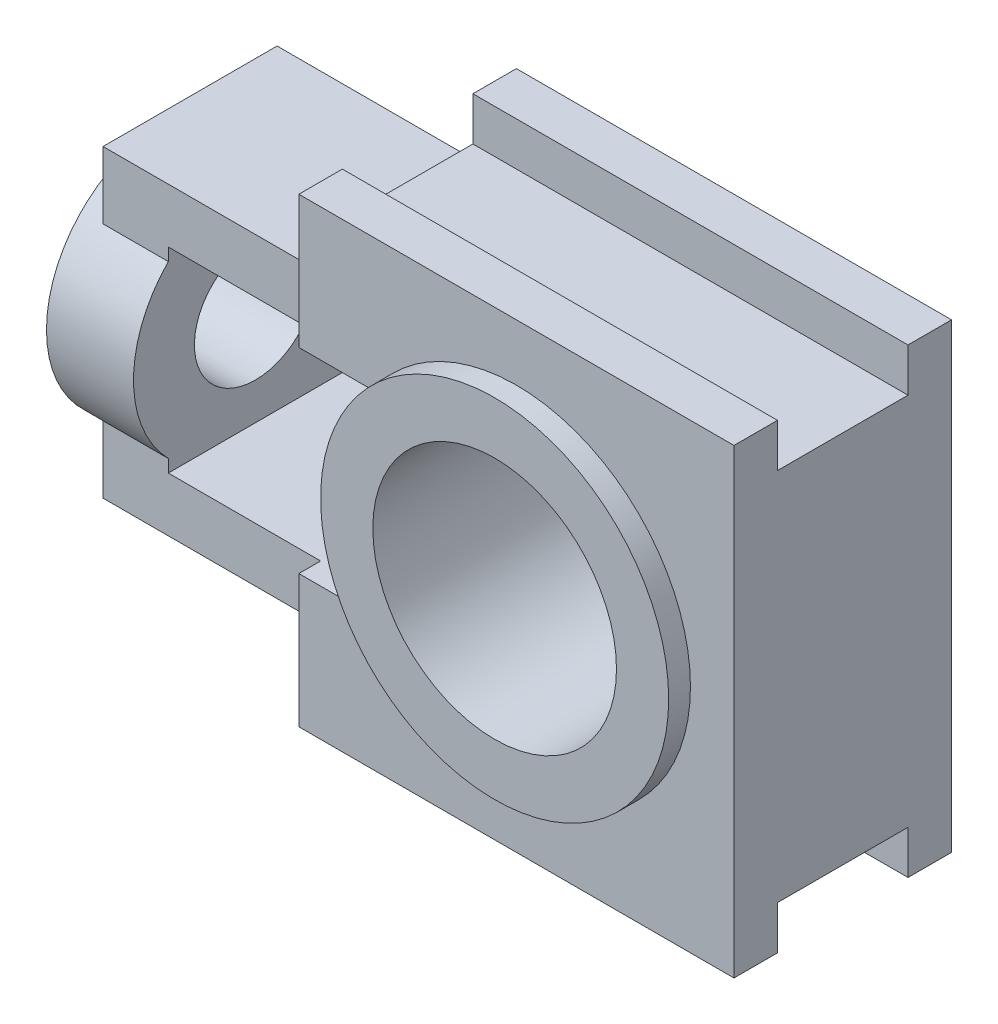
ISO-10303-21;
HEADER;
FILE_DESCRIPTION(('STEP AP214'),'2;1');
FILE_NAME('part.step','',(''),(''),'','','');
FILE_SCHEMA(('AUTOMOTIVE_DESIGN { 1 0 10303 214 1 1 1 1 }'));
ENDSEC;
DATA;
#1=APPLICATION_CONTEXT('core data for automotive mechanical design processes');
#2=APPLICATION_PROTOCOL_DEFINITION('international standard','automotive_design',2000,#1);
#3=PRODUCT_CONTEXT('',#1,'mechanical');
#4=PRODUCT('Part','Part','',(#3));
#5=PRODUCT_RELATED_PRODUCT_CATEGORY('part','',(#4));
#6=PRODUCT_DEFINITION_FORMATION('','',#4);
#7=PRODUCT_DEFINITION_CONTEXT('part definition',#1,'design');
#8=PRODUCT_DEFINITION('design','',#6,#7);
#9=PRODUCT_DEFINITION_SHAPE('','',#8);
#10=(LENGTH_UNIT() NAMED_UNIT(*) SI_UNIT(.MILLI.,.METRE.));
#11=(NAMED_UNIT(*) PLANE_ANGLE_UNIT() SI_UNIT($,.RADIAN.));
#12=(NAMED_UNIT(*) SI_UNIT($,.STERADIAN.) SOLID_ANGLE_UNIT());
#13=UNCERTAINTY_MEASURE_WITH_UNIT(LENGTH_MEASURE(1.E-05),#10,'distance_accuracy_value','');
#14=(GEOMETRIC_REPRESENTATION_CONTEXT(3) GLOBAL_UNCERTAINTY_ASSIGNED_CONTEXT((#13)) GLOBAL_UNIT_ASSIGNED_CONTEXT((#10,
#11,#12)) REPRESENTATION_CONTEXT('',''));
#15=CARTESIAN_POINT('',(0.,0.,0.));
#16=DIRECTION('',(0.,0.,1.));
#17=DIRECTION('',(1.,0.,0.));
#18=AXIS2_PLACEMENT_3D('',#15,#16,#17);
#19=CARTESIAN_POINT('',(0.,0.,20.));
#20=DIRECTION('',(0.,0.,-1.));
#21=DIRECTION('',(-1.,0.,0.));
#22=AXIS2_PLACEMENT_3D('',#19,#20,#21);
#23=PLANE('',#22);
#24=DIRECTION('',(1.,0.,0.));
#25=VECTOR('',#24,1.);
#26=CARTESIAN_POINT('',(-105.,19.5959179422654,20.));
#27=LINE('',#26,#25);
#28=CARTESIAN_POINT('',(-85.,19.5959179422654,20.));
#29=VERTEX_POINT('',#28);
#30=CARTESIAN_POINT('',(-100.,19.5959179422654,20.));
#31=VERTEX_POINT('',#30);
#32=EDGE_CURVE('E348',#29,#31,#27,.F.);
#33=ORIENTED_EDGE('',*,*,#32,.F.);
#34=DIRECTION('',(0.,1.,0.));
#35=VECTOR('',#34,1.);
#36=CARTESIAN_POINT('',(-85.,0.,20.));
#37=LINE('',#36,#35);
#38=CARTESIAN_POINT('',(-85.,22.5,20.));
#39=VERTEX_POINT('',#38);
#40=EDGE_CURVE('E291',#29,#39,#37,.T.);
#41=ORIENTED_EDGE('',*,*,#40,.T.);
#42=DIRECTION('',(1.,0.,0.));
#43=VECTOR('',#42,1.);
#44=CARTESIAN_POINT('',(0.,22.5,20.));
#45=LINE('',#44,#43);
#46=CARTESIAN_POINT('',(-50.,22.5,20.));
#47=VERTEX_POINT('',#46);
#48=EDGE_CURVE('E331',#39,#47,#45,.T.);
#49=ORIENTED_EDGE('',*,*,#48,.T.);
#50=DIRECTION('',(0.,1.,0.));
#51=VECTOR('',#50,1.);
#52=CARTESIAN_POINT('',(-50.,35.,20.));
#53=LINE('',#52,#51);
#54=CARTESIAN_POINT('',(-50.,35.,20.));
#55=VERTEX_POINT('',#54);
#56=EDGE_CURVE('E414',#47,#55,#53,.T.);
#57=ORIENTED_EDGE('',*,*,#56,.T.);
#58=DIRECTION('',(-1.,0.,0.));
#59=VECTOR('',#58,1.);
#60=CARTESIAN_POINT('',(-50.,35.,20.));
#61=LINE('',#60,#59);
#62=CARTESIAN_POINT('',(-100.,35.,20.));
#63=VERTEX_POINT('',#62);
#64=EDGE_CURVE('E413',#55,#63,#61,.T.);
#65=ORIENTED_EDGE('',*,*,#64,.T.);
#66=DIRECTION('',(0.,-1.,0.));
#67=VECTOR('',#66,1.);
#68=CARTESIAN_POINT('',(-100.,35.,20.));
#69=LINE('',#68,#67);
#70=EDGE_CURVE('E417',#63,#31,#69,.T.);
#71=ORIENTED_EDGE('',*,*,#70,.T.);
#72=EDGE_LOOP('',(#33,#41,#49,#57,#65,#71));
#73=FACE_BOUND('',#72,.T.);
#74=ADVANCED_FACE('F44',(#73),#23,.F.);
#75=CARTESIAN_POINT('',(0.,0.,-20.));
#76=DIRECTION('',(0.,0.,-1.));
#77=DIRECTION('',(-1.,0.,0.));
#78=AXIS2_PLACEMENT_3D('',#75,#76,#77);
#79=PLANE('',#78);
#80=DIRECTION('',(0.,1.,0.));
#81=VECTOR('',#80,1.);
#82=CARTESIAN_POINT('',(-85.,0.,-20.));
#83=LINE('',#82,#81);
#84=CARTESIAN_POINT('',(-85.,19.5959179422654,-20.));
#85=VERTEX_POINT('',#84);
#86=CARTESIAN_POINT('',(-85.,22.5,-20.));
#87=VERTEX_POINT('',#86);
#88=EDGE_CURVE('E301',#85,#87,#83,.T.);
#89=ORIENTED_EDGE('',*,*,#88,.F.);
#90=DIRECTION('',(1.,0.,0.));
#91=VECTOR('',#90,1.);
#92=CARTESIAN_POINT('',(-105.,19.5959179422654,-20.));
#93=LINE('',#92,#91);
#94=CARTESIAN_POINT('',(-100.,19.5959179422654,-20.));
#95=VERTEX_POINT('',#94);
#96=EDGE_CURVE('E11',#85,#95,#93,.F.);
#97=ORIENTED_EDGE('',*,*,#96,.T.);
#98=DIRECTION('',(0.,-1.,0.));
#99=VECTOR('',#98,1.);
#100=CARTESIAN_POINT('',(-100.,35.,-20.));
#101=LINE('',#100,#99);
#102=CARTESIAN_POINT('',(-100.,35.,-20.));
#103=VERTEX_POINT('',#102);
#104=EDGE_CURVE('E427',#103,#95,#101,.T.);
#105=ORIENTED_EDGE('',*,*,#104,.F.);
#106=DIRECTION('',(-1.,0.,0.));
#107=VECTOR('',#106,1.);
#108=CARTESIAN_POINT('',(-50.,35.,-20.));
#109=LINE('',#108,#107);
#110=CARTESIAN_POINT('',(-50.,35.,-20.));
#111=VERTEX_POINT('',#110);
#112=EDGE_CURVE('E426',#111,#103,#109,.T.);
#113=ORIENTED_EDGE('',*,*,#112,.F.);
#114=DIRECTION('',(0.,1.,0.));
#115=VECTOR('',#114,1.);
#116=CARTESIAN_POINT('',(-50.,35.,-20.));
#117=LINE('',#116,#115);
#118=CARTESIAN_POINT('',(-50.,22.5,-20.));
#119=VERTEX_POINT('',#118);
#120=EDGE_CURVE('E390',#119,#111,#117,.T.);
#121=ORIENTED_EDGE('',*,*,#120,.F.);
#122=DIRECTION('',(1.,0.,0.));
#123=VECTOR('',#122,1.);
#124=CARTESIAN_POINT('',(0.,22.5,-20.));
#125=LINE('',#124,#123);
#126=EDGE_CURVE('E327',#87,#119,#125,.T.);
#127=ORIENTED_EDGE('',*,*,#126,.F.);
#128=EDGE_LOOP('',(#89,#97,#105,#113,#121,#127));
#129=FACE_BOUND('',#128,.T.);
#130=ADVANCED_FACE('F524',(#129),#79,.T.);
#131=CARTESIAN_POINT('',(-50.,-53.,25.));
#132=DIRECTION('',(1.,0.,0.));
#133=DIRECTION('',(0.,0.,-1.));
#134=AXIS2_PLACEMENT_3D('',#131,#132,#133);
#135=PLANE('',#134);
#136=DIRECTION('',(0.,-1.,0.));
#137=VECTOR('',#136,1.);
#138=CARTESIAN_POINT('',(-50.,-53.,-25.));
#139=LINE('',#138,#137);
#140=CARTESIAN_POINT('',(-50.,53.,-25.));
#141=VERTEX_POINT('',#140);
#142=CARTESIAN_POINT('',(-50.,22.5,-25.));
#143=VERTEX_POINT('',#142);
#144=EDGE_CURVE('E467',#141,#143,#139,.T.);
#145=ORIENTED_EDGE('',*,*,#144,.T.);
#146=DIRECTION('',(0.,0.,1.));
#147=VECTOR('',#146,1.);
#148=CARTESIAN_POINT('',(-50.,22.5,25.));
#149=LINE('',#148,#147);
#150=EDGE_CURVE('E324',#143,#119,#149,.T.);
#151=ORIENTED_EDGE('',*,*,#150,.T.);
#152=ORIENTED_EDGE('',*,*,#120,.T.);
#153=DIRECTION('',(0.,0.,-1.));
#154=VECTOR('',#153,1.);
#155=CARTESIAN_POINT('',(-50.,35.,20.));
#156=LINE('',#155,#154);
#157=EDGE_CURVE('E444',#55,#111,#156,.T.);
#158=ORIENTED_EDGE('',*,*,#157,.F.);
#159=ORIENTED_EDGE('',*,*,#56,.F.);
#160=CARTESIAN_POINT('',(-50.,22.5,25.));
#161=VERTEX_POINT('',#160);
#162=EDGE_CURVE('E328',#47,#161,#149,.T.);
#163=ORIENTED_EDGE('',*,*,#162,.T.);
#164=DIRECTION('',(0.,-1.,0.));
#165=VECTOR('',#164,1.);
#166=CARTESIAN_POINT('',(-50.,-53.,25.));
#167=LINE('',#166,#165);
#168=CARTESIAN_POINT('',(-50.,53.,25.));
#169=VERTEX_POINT('',#168);
#170=EDGE_CURVE('E454',#169,#161,#167,.T.);
#171=ORIENTED_EDGE('',*,*,#170,.F.);
#172=DIRECTION('',(0.,0.,-1.));
#173=VECTOR('',#172,1.);
#174=CARTESIAN_POINT('',(-50.,53.,25.));
#175=LINE('',#174,#173);
#176=CARTESIAN_POINT('',(-50.,53.,15.));
#177=VERTEX_POINT('',#176);
#178=EDGE_CURVE('E479',#169,#177,#175,.T.);
#179=ORIENTED_EDGE('',*,*,#178,.T.);
#180=DIRECTION('',(0.,1.,0.));
#181=VECTOR('',#180,1.);
#182=CARTESIAN_POINT('',(-50.,53.,15.));
#183=LINE('',#182,#181);
#184=CARTESIAN_POINT('',(-50.,43.,15.));
#185=VERTEX_POINT('',#184);
#186=EDGE_CURVE('E374',#185,#177,#183,.T.);
#187=ORIENTED_EDGE('',*,*,#186,.F.);
#188=DIRECTION('',(0.,0.,1.));
#189=VECTOR('',#188,1.);
#190=CARTESIAN_POINT('',(-50.,43.,-15.));
#191=LINE('',#190,#189);
#192=CARTESIAN_POINT('',(-50.,43.,-15.));
#193=VERTEX_POINT('',#192);
#194=EDGE_CURVE('E371',#193,#185,#191,.T.);
#195=ORIENTED_EDGE('',*,*,#194,.F.);
#196=DIRECTION('',(0.,-1.,0.));
#197=VECTOR('',#196,1.);
#198=CARTESIAN_POINT('',(-50.,53.,-15.));
#199=LINE('',#198,#197);
#200=CARTESIAN_POINT('',(-50.,53.,-15.));
#201=VERTEX_POINT('',#200);
#202=EDGE_CURVE('E369',#201,#193,#199,.T.);
#203=ORIENTED_EDGE('',*,*,#202,.F.);
#204=EDGE_CURVE('E476',#201,#141,#175,.T.);
#205=ORIENTED_EDGE('',*,*,#204,.T.);
#206=EDGE_LOOP('',(#145,#151,#152,#158,#159,#163,#171,#179,#187,#195,#203,#205));
#207=FACE_BOUND('',#206,.T.);
#208=ADVANCED_FACE('F590',(#207),#135,.F.);
#209=CARTESIAN_POINT('',(-100.,35.,20.));
#210=DIRECTION('',(1.,0.,0.));
#211=DIRECTION('',(0.,0.,-1.));
#212=AXIS2_PLACEMENT_3D('',#209,#210,#211);
#213=PLANE('',#212);
#214=CARTESIAN_POINT('',(-100.,0.,0.));
#215=DIRECTION('',(1.,0.,0.));
#216=DIRECTION('',(0.,0.,-1.));
#217=AXIS2_PLACEMENT_3D('',#214,#215,#216);
#218=CIRCLE('',#217,28.);
#219=CARTESIAN_POINT('',(-100.,-19.5959179422654,-20.));
#220=VERTEX_POINT('',#219);
#221=CARTESIAN_POINT('',(-100.,-19.5959179422654,20.));
#222=VERTEX_POINT('',#221);
#223=EDGE_CURVE('E344',#220,#222,#218,.F.);
#224=ORIENTED_EDGE('',*,*,#223,.F.);
#225=CARTESIAN_POINT('',(-100.,-35.,-20.));
#226=VERTEX_POINT('',#225);
#227=EDGE_CURVE('E428',#220,#226,#101,.T.);
#228=ORIENTED_EDGE('',*,*,#227,.T.);
#229=DIRECTION('',(0.,0.,-1.));
#230=VECTOR('',#229,1.);
#231=CARTESIAN_POINT('',(-100.,-35.,20.));
#232=LINE('',#231,#230);
#233=CARTESIAN_POINT('',(-100.,-35.,20.));
#234=VERTEX_POINT('',#233);
#235=EDGE_CURVE('E440',#234,#226,#232,.T.);
#236=ORIENTED_EDGE('',*,*,#235,.F.);
#237=EDGE_CURVE('E418',#222,#234,#69,.T.);
#238=ORIENTED_EDGE('',*,*,#237,.F.);
#239=EDGE_LOOP('',(#224,#228,#236,#238));
#240=FACE_BOUND('',#239,.T.);
#241=ADVANCED_FACE('F505',(#240),#213,.F.);
#242=DIRECTION('',(-1.,0.,0.));
#243=VECTOR('',#242,1.);
#244=CARTESIAN_POINT('',(0.,-22.5,20.));
#245=LINE('',#244,#243);
#246=CARTESIAN_POINT('',(-50.,-22.5,20.));
#247=VERTEX_POINT('',#246);
#248=CARTESIAN_POINT('',(-85.,-22.5,20.));
#249=VERTEX_POINT('',#248);
#250=EDGE_CURVE('E319',#247,#249,#245,.T.);
#251=ORIENTED_EDGE('',*,*,#250,.T.);
#252=CARTESIAN_POINT('',(-85.,-19.5959179422654,20.));
#253=VERTEX_POINT('',#252);
#254=EDGE_CURVE('E308',#249,#253,#37,.T.);
#255=ORIENTED_EDGE('',*,*,#254,.T.);
#256=DIRECTION('',(1.,0.,0.));
#257=VECTOR('',#256,1.);
#258=CARTESIAN_POINT('',(-105.,-19.5959179422654,20.));
#259=LINE('',#258,#257);
#260=EDGE_CURVE('E347',#222,#253,#259,.T.);
#261=ORIENTED_EDGE('',*,*,#260,.F.);
#262=ORIENTED_EDGE('',*,*,#237,.T.);
#263=DIRECTION('',(1.,0.,0.));
#264=VECTOR('',#263,1.);
#265=CARTESIAN_POINT('',(-50.,-35.,20.));
#266=LINE('',#265,#264);
#267=CARTESIAN_POINT('',(-50.,-35.,20.));
#268=VERTEX_POINT('',#267);
#269=EDGE_CURVE('E419',#234,#268,#266,.T.);
#270=ORIENTED_EDGE('',*,*,#269,.T.);
#271=EDGE_CURVE('E407',#268,#247,#53,.T.);
#272=ORIENTED_EDGE('',*,*,#271,.T.);
#273=EDGE_LOOP('',(#251,#255,#261,#262,#270,#272));
#274=FACE_BOUND('',#273,.T.);
#275=ADVANCED_FACE('F507',(#274),#23,.F.);
#276=CARTESIAN_POINT('',(-85.,-22.5,-20.));
#277=VERTEX_POINT('',#276);
#278=CARTESIAN_POINT('',(-85.,-19.5959179422654,-20.));
#279=VERTEX_POINT('',#278);
#280=EDGE_CURVE('E306',#277,#279,#83,.T.);
#281=ORIENTED_EDGE('',*,*,#280,.F.);
#282=DIRECTION('',(-1.,0.,0.));
#283=VECTOR('',#282,1.);
#284=CARTESIAN_POINT('',(0.,-22.5,-20.));
#285=LINE('',#284,#283);
#286=CARTESIAN_POINT('',(-50.,-22.5,-20.));
#287=VERTEX_POINT('',#286);
#288=EDGE_CURVE('E314',#287,#277,#285,.T.);
#289=ORIENTED_EDGE('',*,*,#288,.F.);
#290=CARTESIAN_POINT('',(-50.,-35.,-20.));
#291=VERTEX_POINT('',#290);
#292=EDGE_CURVE('E421',#291,#287,#117,.T.);
#293=ORIENTED_EDGE('',*,*,#292,.F.);
#294=DIRECTION('',(1.,0.,0.));
#295=VECTOR('',#294,1.);
#296=CARTESIAN_POINT('',(-50.,-35.,-20.));
#297=LINE('',#296,#295);
#298=EDGE_CURVE('E435',#226,#291,#297,.T.);
#299=ORIENTED_EDGE('',*,*,#298,.F.);
#300=ORIENTED_EDGE('',*,*,#227,.F.);
#301=DIRECTION('',(1.,0.,0.));
#302=VECTOR('',#301,1.);
#303=CARTESIAN_POINT('',(-105.,-19.5959179422654,-20.));
#304=LINE('',#303,#302);
#305=EDGE_CURVE('E52',#220,#279,#304,.T.);
#306=ORIENTED_EDGE('',*,*,#305,.T.);
#307=EDGE_LOOP('',(#281,#289,#293,#299,#300,#306));
#308=FACE_BOUND('',#307,.T.);
#309=ADVANCED_FACE('F489',(#308),#79,.T.);
#310=CARTESIAN_POINT('',(-50.,53.,25.));
#311=DIRECTION('',(0.,-1.,0.));
#312=DIRECTION('',(0.,0.,-1.));
#313=AXIS2_PLACEMENT_3D('',#310,#311,#312);
#314=PLANE('',#313);
#315=ORIENTED_EDGE('',*,*,#204,.F.);
#316=DIRECTION('',(-1.,0.,0.));
#317=VECTOR('',#316,1.);
#318=CARTESIAN_POINT('',(81.6227766016838,53.,-15.));
#319=LINE('',#318,#317);
#320=CARTESIAN_POINT('',(50.,53.,-15.));
#321=VERTEX_POINT('',#320);
#322=EDGE_CURVE('E368',#321,#201,#319,.T.);
#323=ORIENTED_EDGE('',*,*,#322,.F.);
#324=DIRECTION('',(0.,0.,-1.));
#325=VECTOR('',#324,1.);
#326=CARTESIAN_POINT('',(50.,53.,25.));
#327=LINE('',#326,#325);
#328=CARTESIAN_POINT('',(50.,53.,-25.));
#329=VERTEX_POINT('',#328);
#330=EDGE_CURVE('E485',#321,#329,#327,.T.);
#331=ORIENTED_EDGE('',*,*,#330,.T.);
#332=DIRECTION('',(-1.,0.,0.));
#333=VECTOR('',#332,1.);
#334=CARTESIAN_POINT('',(-50.,53.,-25.));
#335=LINE('',#334,#333);
#336=EDGE_CURVE('E465',#329,#141,#335,.T.);
#337=ORIENTED_EDGE('',*,*,#336,.T.);
#338=EDGE_LOOP('',(#315,#323,#331,#337));
#339=FACE_BOUND('',#338,.T.);
#340=ADVANCED_FACE('F598',(#339),#314,.F.);
#341=CARTESIAN_POINT('',(-50.,-53.,25.));
#342=DIRECTION('',(0.,1.,0.));
#343=DIRECTION('',(0.,0.,1.));
#344=AXIS2_PLACEMENT_3D('',#341,#342,#343);
#345=PLANE('',#344);
#346=DIRECTION('',(0.,0.,-1.));
#347=VECTOR('',#346,1.);
#348=CARTESIAN_POINT('',(50.,-53.,25.));
#349=LINE('',#348,#347);
#350=CARTESIAN_POINT('',(50.,-53.,-15.));
#351=VERTEX_POINT('',#350);
#352=CARTESIAN_POINT('',(50.,-53.,-25.));
#353=VERTEX_POINT('',#352);
#354=EDGE_CURVE('E459',#351,#353,#349,.T.);
#355=ORIENTED_EDGE('',*,*,#354,.F.);
#356=DIRECTION('',(-1.,0.,0.));
#357=VECTOR('',#356,1.);
#358=CARTESIAN_POINT('',(81.6227766016838,-53.,-15.));
#359=LINE('',#358,#357);
#360=CARTESIAN_POINT('',(-50.,-53.,-15.));
#361=VERTEX_POINT('',#360);
#362=EDGE_CURVE('E393',#351,#361,#359,.T.);
#363=ORIENTED_EDGE('',*,*,#362,.T.);
#364=DIRECTION('',(0.,0.,-1.));
#365=VECTOR('',#364,1.);
#366=CARTESIAN_POINT('',(-50.,-53.,25.));
#367=LINE('',#366,#365);
#368=CARTESIAN_POINT('',(-50.,-53.,-25.));
#369=VERTEX_POINT('',#368);
#370=EDGE_CURVE('E475',#361,#369,#367,.T.);
#371=ORIENTED_EDGE('',*,*,#370,.T.);
#372=DIRECTION('',(1.,0.,0.));
#373=VECTOR('',#372,1.);
#374=CARTESIAN_POINT('',(-50.,-53.,-25.));
#375=LINE('',#374,#373);
#376=EDGE_CURVE('E452',#369,#353,#375,.T.);
#377=ORIENTED_EDGE('',*,*,#376,.T.);
#378=EDGE_LOOP('',(#355,#363,#371,#377));
#379=FACE_BOUND('',#378,.T.);
#380=ADVANCED_FACE('F553',(#379),#345,.F.);
#381=CARTESIAN_POINT('',(50.,-53.,25.));
#382=DIRECTION('',(-1.,0.,0.));
#383=DIRECTION('',(0.,0.,1.));
#384=AXIS2_PLACEMENT_3D('',#381,#382,#383);
#385=PLANE('',#384);
#386=ORIENTED_EDGE('',*,*,#330,.F.);
#387=DIRECTION('',(0.,1.,0.));
#388=VECTOR('',#387,1.);
#389=CARTESIAN_POINT('',(50.,53.,-15.));
#390=LINE('',#389,#388);
#391=CARTESIAN_POINT('',(50.,43.,-15.));
#392=VERTEX_POINT('',#391);
#393=EDGE_CURVE('E364',#392,#321,#390,.T.);
#394=ORIENTED_EDGE('',*,*,#393,.F.);
#395=DIRECTION('',(0.,0.,-1.));
#396=VECTOR('',#395,1.);
#397=CARTESIAN_POINT('',(50.,43.,-15.));
#398=LINE('',#397,#396);
#399=CARTESIAN_POINT('',(50.,43.,15.));
#400=VERTEX_POINT('',#399);
#401=EDGE_CURVE('E366',#400,#392,#398,.T.);
#402=ORIENTED_EDGE('',*,*,#401,.F.);
#403=DIRECTION('',(0.,-1.,0.));
#404=VECTOR('',#403,1.);
#405=CARTESIAN_POINT('',(50.,53.,15.));
#406=LINE('',#405,#404);
#407=CARTESIAN_POINT('',(50.,53.,15.));
#408=VERTEX_POINT('',#407);
#409=EDGE_CURVE('E361',#408,#400,#406,.T.);
#410=ORIENTED_EDGE('',*,*,#409,.F.);
#411=CARTESIAN_POINT('',(50.,53.,25.));
#412=VERTEX_POINT('',#411);
#413=EDGE_CURVE('E362',#412,#408,#327,.T.);
#414=ORIENTED_EDGE('',*,*,#413,.F.);
#415=DIRECTION('',(0.,1.,0.));
#416=VECTOR('',#415,1.);
#417=CARTESIAN_POINT('',(50.,-53.,25.));
#418=LINE('',#417,#416);
#419=CARTESIAN_POINT('',(50.,-53.,25.));
#420=VERTEX_POINT('',#419);
#421=EDGE_CURVE('E450',#420,#412,#418,.T.);
#422=ORIENTED_EDGE('',*,*,#421,.F.);
#423=CARTESIAN_POINT('',(50.,-53.,15.));
#424=VERTEX_POINT('',#423);
#425=EDGE_CURVE('E473',#420,#424,#349,.T.);
#426=ORIENTED_EDGE('',*,*,#425,.T.);
#427=DIRECTION('',(0.,-1.,0.));
#428=VECTOR('',#427,1.);
#429=CARTESIAN_POINT('',(50.,-53.,15.));
#430=LINE('',#429,#428);
#431=CARTESIAN_POINT('',(50.,-43.,15.));
#432=VERTEX_POINT('',#431);
#433=EDGE_CURVE('E375',#432,#424,#430,.T.);
#434=ORIENTED_EDGE('',*,*,#433,.F.);
#435=DIRECTION('',(0.,0.,1.));
#436=VECTOR('',#435,1.);
#437=CARTESIAN_POINT('',(50.,-43.,-15.));
#438=LINE('',#437,#436);
#439=CARTESIAN_POINT('',(50.,-43.,-15.));
#440=VERTEX_POINT('',#439);
#441=EDGE_CURVE('E389',#440,#432,#438,.T.);
#442=ORIENTED_EDGE('',*,*,#441,.F.);
#443=DIRECTION('',(0.,1.,0.));
#444=VECTOR('',#443,1.);
#445=CARTESIAN_POINT('',(50.,-53.,-15.));
#446=LINE('',#445,#444);
#447=EDGE_CURVE('E388',#351,#440,#446,.T.);
#448=ORIENTED_EDGE('',*,*,#447,.F.);
#449=ORIENTED_EDGE('',*,*,#354,.T.);
#450=DIRECTION('',(0.,1.,0.));
#451=VECTOR('',#450,1.);
#452=CARTESIAN_POINT('',(50.,-53.,-25.));
#453=LINE('',#452,#451);
#454=EDGE_CURVE('E448',#353,#329,#453,.T.);
#455=ORIENTED_EDGE('',*,*,#454,.T.);
#456=EDGE_LOOP('',(#386,#394,#402,#410,#414,#422,#426,#434,#442,#448,#449,#455));
#457=FACE_BOUND('',#456,.T.);
#458=ADVANCED_FACE('F50',(#457),#385,.F.);
#459=ORIENTED_EDGE('',*,*,#413,.T.);
#460=DIRECTION('',(-1.,0.,0.));
#461=VECTOR('',#460,1.);
#462=CARTESIAN_POINT('',(81.6227766016838,53.,15.));
#463=LINE('',#462,#461);
#464=EDGE_CURVE('E377',#408,#177,#463,.T.);
#465=ORIENTED_EDGE('',*,*,#464,.T.);
#466=ORIENTED_EDGE('',*,*,#178,.F.);
#467=DIRECTION('',(-1.,0.,0.));
#468=VECTOR('',#467,1.);
#469=CARTESIAN_POINT('',(-50.,53.,25.));
#470=LINE('',#469,#468);
#471=EDGE_CURVE('E447',#412,#169,#470,.T.);
#472=ORIENTED_EDGE('',*,*,#471,.F.);
#473=EDGE_LOOP('',(#459,#465,#466,#472));
#474=FACE_BOUND('',#473,.T.);
#475=ADVANCED_FACE('F582',(#474),#314,.F.);
#476=CARTESIAN_POINT('',(-50.,-22.5,25.));
#477=VERTEX_POINT('',#476);
#478=CARTESIAN_POINT('',(-50.,-53.,25.));
#479=VERTEX_POINT('',#478);
#480=EDGE_CURVE('E453',#477,#479,#167,.T.);
#481=ORIENTED_EDGE('',*,*,#480,.F.);
#482=DIRECTION('',(0.,0.,-1.));
#483=VECTOR('',#482,1.);
#484=CARTESIAN_POINT('',(-50.,-22.5,25.));
#485=LINE('',#484,#483);
#486=EDGE_CURVE('E312',#477,#247,#485,.T.);
#487=ORIENTED_EDGE('',*,*,#486,.T.);
#488=ORIENTED_EDGE('',*,*,#271,.F.);
#489=DIRECTION('',(0.,0.,-1.));
#490=VECTOR('',#489,1.);
#491=CARTESIAN_POINT('',(-50.,-35.,20.));
#492=LINE('',#491,#490);
#493=EDGE_CURVE('E425',#268,#291,#492,.T.);
#494=ORIENTED_EDGE('',*,*,#493,.T.);
#495=ORIENTED_EDGE('',*,*,#292,.T.);
#496=CARTESIAN_POINT('',(-50.,-22.5,-25.));
#497=VERTEX_POINT('',#496);
#498=EDGE_CURVE('E313',#287,#497,#485,.T.);
#499=ORIENTED_EDGE('',*,*,#498,.T.);
#500=EDGE_CURVE('E462',#497,#369,#139,.T.);
#501=ORIENTED_EDGE('',*,*,#500,.T.);
#502=ORIENTED_EDGE('',*,*,#370,.F.);
#503=DIRECTION('',(0.,-1.,0.));
#504=VECTOR('',#503,1.);
#505=CARTESIAN_POINT('',(-50.,-53.,-15.));
#506=LINE('',#505,#504);
#507=CARTESIAN_POINT('',(-50.,-43.,-15.));
#508=VERTEX_POINT('',#507);
#509=EDGE_CURVE('E399',#508,#361,#506,.T.);
#510=ORIENTED_EDGE('',*,*,#509,.F.);
#511=DIRECTION('',(0.,0.,-1.));
#512=VECTOR('',#511,1.);
#513=CARTESIAN_POINT('',(-50.,-43.,-15.));
#514=LINE('',#513,#512);
#515=CARTESIAN_POINT('',(-50.,-43.,15.));
#516=VERTEX_POINT('',#515);
#517=EDGE_CURVE('E397',#516,#508,#514,.T.);
#518=ORIENTED_EDGE('',*,*,#517,.F.);
#519=DIRECTION('',(0.,1.,0.));
#520=VECTOR('',#519,1.);
#521=CARTESIAN_POINT('',(-50.,-53.,15.));
#522=LINE('',#521,#520);
#523=CARTESIAN_POINT('',(-50.,-53.,15.));
#524=VERTEX_POINT('',#523);
#525=EDGE_CURVE('E391',#524,#516,#522,.T.);
#526=ORIENTED_EDGE('',*,*,#525,.F.);
#527=EDGE_CURVE('E474',#479,#524,#367,.T.);
#528=ORIENTED_EDGE('',*,*,#527,.F.);
#529=EDGE_LOOP('',(#481,#487,#488,#494,#495,#499,#501,#502,#510,#518,#526,#528));
#530=FACE_BOUND('',#529,.T.);
#531=ADVANCED_FACE('F531',(#530),#135,.F.);
#532=ORIENTED_EDGE('',*,*,#527,.T.);
#533=DIRECTION('',(-1.,0.,0.));
#534=VECTOR('',#533,1.);
#535=CARTESIAN_POINT('',(81.6227766016838,-53.,15.));
#536=LINE('',#535,#534);
#537=EDGE_CURVE('E402',#424,#524,#536,.T.);
#538=ORIENTED_EDGE('',*,*,#537,.F.);
#539=ORIENTED_EDGE('',*,*,#425,.F.);
#540=DIRECTION('',(1.,0.,0.));
#541=VECTOR('',#540,1.);
#542=CARTESIAN_POINT('',(-50.,-53.,25.));
#543=LINE('',#542,#541);
#544=EDGE_CURVE('E460',#479,#420,#543,.T.);
#545=ORIENTED_EDGE('',*,*,#544,.F.);
#546=EDGE_LOOP('',(#532,#538,#539,#545));
#547=FACE_BOUND('',#546,.T.);
#548=ADVANCED_FACE('F574',(#547),#345,.F.);
#549=CARTESIAN_POINT('',(0.,0.,25.));
#550=DIRECTION('',(0.,0.,-1.));
#551=DIRECTION('',(-1.,0.,0.));
#552=AXIS2_PLACEMENT_3D('',#549,#550,#551);
#553=PLANE('',#552);
#554=ORIENTED_EDGE('',*,*,#170,.T.);
#555=DIRECTION('',(1.,0.,0.));
#556=VECTOR('',#555,1.);
#557=CARTESIAN_POINT('',(0.,22.5,25.));
#558=LINE('',#557,#556);
#559=CARTESIAN_POINT('',(-33.0718913883074,22.5,25.));
#560=VERTEX_POINT('',#559);
#561=EDGE_CURVE('E332',#161,#560,#558,.T.);
#562=ORIENTED_EDGE('',*,*,#561,.T.);
#563=CARTESIAN_POINT('',(0.,0.,25.));
#564=DIRECTION('',(0.,0.,-1.));
#565=DIRECTION('',(-1.,0.,0.));
#566=AXIS2_PLACEMENT_3D('',#563,#564,#565);
#567=CIRCLE('',#566,40.);
#568=CARTESIAN_POINT('',(-33.0718913883074,-22.5,25.));
#569=VERTEX_POINT('',#568);
#570=EDGE_CURVE('E359',#569,#560,#567,.F.);
#571=ORIENTED_EDGE('',*,*,#570,.F.);
#572=DIRECTION('',(-1.,0.,0.));
#573=VECTOR('',#572,1.);
#574=CARTESIAN_POINT('',(0.,-22.5,25.));
#575=LINE('',#574,#573);
#576=EDGE_CURVE('E320',#569,#477,#575,.T.);
#577=ORIENTED_EDGE('',*,*,#576,.T.);
#578=ORIENTED_EDGE('',*,*,#480,.T.);
#579=ORIENTED_EDGE('',*,*,#544,.T.);
#580=ORIENTED_EDGE('',*,*,#421,.T.);
#581=ORIENTED_EDGE('',*,*,#471,.T.);
#582=EDGE_LOOP('',(#554,#562,#571,#577,#578,#579,#580,#581));
#583=FACE_BOUND('',#582,.T.);
#584=ADVANCED_FACE('F540',(#583),#553,.F.);
#585=CARTESIAN_POINT('',(0.,0.,-25.));
#586=DIRECTION('',(0.,0.,-1.));
#587=DIRECTION('',(-1.,0.,0.));
#588=AXIS2_PLACEMENT_3D('',#585,#586,#587);
#589=PLANE('',#588);
#590=DIRECTION('',(1.,0.,0.));
#591=VECTOR('',#590,1.);
#592=CARTESIAN_POINT('',(0.,22.5,-25.));
#593=LINE('',#592,#591);
#594=CARTESIAN_POINT('',(-33.0718913883074,22.5,-25.));
#595=VERTEX_POINT('',#594);
#596=EDGE_CURVE('E323',#143,#595,#593,.T.);
#597=ORIENTED_EDGE('',*,*,#596,.F.);
#598=ORIENTED_EDGE('',*,*,#144,.F.);
#599=ORIENTED_EDGE('',*,*,#336,.F.);
#600=ORIENTED_EDGE('',*,*,#454,.F.);
#601=ORIENTED_EDGE('',*,*,#376,.F.);
#602=ORIENTED_EDGE('',*,*,#500,.F.);
#603=DIRECTION('',(-1.,0.,0.));
#604=VECTOR('',#603,1.);
#605=CARTESIAN_POINT('',(0.,-22.5,-25.));
#606=LINE('',#605,#604);
#607=CARTESIAN_POINT('',(-33.0718913883074,-22.5,-25.));
#608=VERTEX_POINT('',#607);
#609=EDGE_CURVE('E310',#608,#497,#606,.T.);
#610=ORIENTED_EDGE('',*,*,#609,.F.);
#611=CARTESIAN_POINT('',(0.,0.,-25.));
#612=DIRECTION('',(0.,0.,-1.));
#613=DIRECTION('',(-1.,0.,0.));
#614=AXIS2_PLACEMENT_3D('',#611,#612,#613);
#615=CIRCLE('',#614,40.);
#616=EDGE_CURVE('E357',#608,#595,#615,.F.);
#617=ORIENTED_EDGE('',*,*,#616,.T.);
#618=EDGE_LOOP('',(#597,#598,#599,#600,#601,#602,#610,#617));
#619=FACE_BOUND('',#618,.T.);
#620=ADVANCED_FACE('F550',(#619),#589,.T.);
#621=CARTESIAN_POINT('',(-50.,35.,20.));
#622=DIRECTION('',(0.,-1.,0.));
#623=DIRECTION('',(1.,0.,0.));
#624=AXIS2_PLACEMENT_3D('',#621,#622,#623);
#625=PLANE('',#624);
#626=ORIENTED_EDGE('',*,*,#112,.T.);
#627=DIRECTION('',(0.,0.,-1.));
#628=VECTOR('',#627,1.);
#629=CARTESIAN_POINT('',(-100.,35.,20.));
#630=LINE('',#629,#628);
#631=EDGE_CURVE('E439',#63,#103,#630,.T.);
#632=ORIENTED_EDGE('',*,*,#631,.F.);
#633=ORIENTED_EDGE('',*,*,#64,.F.);
#634=ORIENTED_EDGE('',*,*,#157,.T.);
#635=EDGE_LOOP('',(#626,#632,#633,#634));
#636=FACE_BOUND('',#635,.T.);
#637=ADVANCED_FACE('F640',(#636),#625,.F.);
#638=EDGE_CURVE('E350',#31,#95,#218,.F.);
#639=ORIENTED_EDGE('',*,*,#638,.F.);
#640=ORIENTED_EDGE('',*,*,#70,.F.);
#641=ORIENTED_EDGE('',*,*,#631,.T.);
#642=ORIENTED_EDGE('',*,*,#104,.T.);
#643=EDGE_LOOP('',(#639,#640,#641,#642));
#644=FACE_BOUND('',#643,.T.);
#645=ADVANCED_FACE('F519',(#644),#213,.F.);
#646=CARTESIAN_POINT('',(-50.,-35.,20.));
#647=DIRECTION('',(0.,1.,0.));
#648=DIRECTION('',(-1.,0.,0.));
#649=AXIS2_PLACEMENT_3D('',#646,#647,#648);
#650=PLANE('',#649);
#651=ORIENTED_EDGE('',*,*,#298,.T.);
#652=ORIENTED_EDGE('',*,*,#493,.F.);
#653=ORIENTED_EDGE('',*,*,#269,.F.);
#654=ORIENTED_EDGE('',*,*,#235,.T.);
#655=EDGE_LOOP('',(#651,#652,#653,#654));
#656=FACE_BOUND('',#655,.T.);
#657=ADVANCED_FACE('F636',(#656),#650,.F.);
#658=CARTESIAN_POINT('',(81.6227766016838,-53.,-15.));
#659=DIRECTION('',(0.,0.,-1.));
#660=DIRECTION('',(0.,1.,0.));
#661=AXIS2_PLACEMENT_3D('',#658,#659,#660);
#662=PLANE('',#661);
#663=ORIENTED_EDGE('',*,*,#447,.T.);
#664=DIRECTION('',(-1.,0.,0.));
#665=VECTOR('',#664,1.);
#666=CARTESIAN_POINT('',(81.6227766016838,-43.,-15.));
#667=LINE('',#666,#665);
#668=EDGE_CURVE('E404',#440,#508,#667,.T.);
#669=ORIENTED_EDGE('',*,*,#668,.T.);
#670=ORIENTED_EDGE('',*,*,#509,.T.);
#671=ORIENTED_EDGE('',*,*,#362,.F.);
#672=EDGE_LOOP('',(#663,#669,#670,#671));
#673=FACE_BOUND('',#672,.T.);
#674=ADVANCED_FACE('F556',(#673),#662,.F.);
#675=CARTESIAN_POINT('',(81.6227766016838,-43.,-15.));
#676=DIRECTION('',(0.,1.,0.));
#677=DIRECTION('',(0.,0.,1.));
#678=AXIS2_PLACEMENT_3D('',#675,#676,#677);
#679=PLANE('',#678);
#680=ORIENTED_EDGE('',*,*,#441,.T.);
#681=DIRECTION('',(-1.,0.,0.));
#682=VECTOR('',#681,1.);
#683=CARTESIAN_POINT('',(81.6227766016838,-43.,15.));
#684=LINE('',#683,#682);
#685=EDGE_CURVE('E408',#432,#516,#684,.T.);
#686=ORIENTED_EDGE('',*,*,#685,.T.);
#687=ORIENTED_EDGE('',*,*,#517,.T.);
#688=ORIENTED_EDGE('',*,*,#668,.F.);
#689=EDGE_LOOP('',(#680,#686,#687,#688));
#690=FACE_BOUND('',#689,.T.);
#691=ADVANCED_FACE('F567',(#690),#679,.F.);
#692=CARTESIAN_POINT('',(81.6227766016838,-53.,15.));
#693=DIRECTION('',(0.,0.,1.));
#694=DIRECTION('',(0.,-1.,0.));
#695=AXIS2_PLACEMENT_3D('',#692,#693,#694);
#696=PLANE('',#695);
#697=ORIENTED_EDGE('',*,*,#433,.T.);
#698=ORIENTED_EDGE('',*,*,#537,.T.);
#699=ORIENTED_EDGE('',*,*,#525,.T.);
#700=ORIENTED_EDGE('',*,*,#685,.F.);
#701=EDGE_LOOP('',(#697,#698,#699,#700));
#702=FACE_BOUND('',#701,.T.);
#703=ADVANCED_FACE('F566',(#702),#696,.F.);
#704=CARTESIAN_POINT('',(81.6227766016838,53.,-15.));
#705=DIRECTION('',(0.,0.,-1.));
#706=DIRECTION('',(0.,1.,0.));
#707=AXIS2_PLACEMENT_3D('',#704,#705,#706);
#708=PLANE('',#707);
#709=ORIENTED_EDGE('',*,*,#393,.T.);
#710=ORIENTED_EDGE('',*,*,#322,.T.);
#711=ORIENTED_EDGE('',*,*,#202,.T.);
#712=DIRECTION('',(-1.,0.,0.));
#713=VECTOR('',#712,1.);
#714=CARTESIAN_POINT('',(81.6227766016838,43.,-15.));
#715=LINE('',#714,#713);
#716=EDGE_CURVE('E380',#392,#193,#715,.T.);
#717=ORIENTED_EDGE('',*,*,#716,.F.);
#718=EDGE_LOOP('',(#709,#710,#711,#717));
#719=FACE_BOUND('',#718,.T.);
#720=ADVANCED_FACE('F605',(#719),#708,.F.);
#721=CARTESIAN_POINT('',(81.6227766016838,53.,15.));
#722=DIRECTION('',(0.,0.,1.));
#723=DIRECTION('',(0.,-1.,0.));
#724=AXIS2_PLACEMENT_3D('',#721,#722,#723);
#725=PLANE('',#724);
#726=ORIENTED_EDGE('',*,*,#409,.T.);
#727=DIRECTION('',(-1.,0.,0.));
#728=VECTOR('',#727,1.);
#729=CARTESIAN_POINT('',(81.6227766016838,43.,15.));
#730=LINE('',#729,#728);
#731=EDGE_CURVE('E385',#400,#185,#730,.T.);
#732=ORIENTED_EDGE('',*,*,#731,.T.);
#733=ORIENTED_EDGE('',*,*,#186,.T.);
#734=ORIENTED_EDGE('',*,*,#464,.F.);
#735=EDGE_LOOP('',(#726,#732,#733,#734));
#736=FACE_BOUND('',#735,.T.);
#737=ADVANCED_FACE('F610',(#736),#725,.F.);
#738=CARTESIAN_POINT('',(81.6227766016838,43.,-15.));
#739=DIRECTION('',(0.,-1.,0.));
#740=DIRECTION('',(0.,0.,-1.));
#741=AXIS2_PLACEMENT_3D('',#738,#739,#740);
#742=PLANE('',#741);
#743=ORIENTED_EDGE('',*,*,#401,.T.);
#744=ORIENTED_EDGE('',*,*,#716,.T.);
#745=ORIENTED_EDGE('',*,*,#194,.T.);
#746=ORIENTED_EDGE('',*,*,#731,.F.);
#747=EDGE_LOOP('',(#743,#744,#745,#746));
#748=FACE_BOUND('',#747,.T.);
#749=ADVANCED_FACE('F603',(#748),#742,.F.);
#750=CARTESIAN_POINT('',(0.,0.,-30.));
#751=DIRECTION('',(0.,0.,1.));
#752=DIRECTION('',(1.,0.,0.));
#753=AXIS2_PLACEMENT_3D('',#750,#751,#752);
#754=PLANE('',#753);
#755=CARTESIAN_POINT('',(0.,0.,-30.));
#756=DIRECTION('',(0.,0.,1.));
#757=DIRECTION('',(1.,0.,0.));
#758=AXIS2_PLACEMENT_3D('',#755,#756,#757);
#759=CIRCLE('',#758,28.);
#760=CARTESIAN_POINT('',(28.,0.,-30.));
#761=VERTEX_POINT('',#760);
#762=EDGE_CURVE('E289',#761,#761,#759,.T.);
#763=ORIENTED_EDGE('',*,*,#762,.T.);
#764=EDGE_LOOP('',(#763));
#765=FACE_BOUND('',#764,.T.);
#766=CARTESIAN_POINT('',(0.,0.,-30.));
#767=DIRECTION('',(0.,0.,1.));
#768=DIRECTION('',(1.,0.,0.));
#769=AXIS2_PLACEMENT_3D('',#766,#767,#768);
#770=CIRCLE('',#769,40.);
#771=CARTESIAN_POINT('',(40.,0.,-30.));
#772=VERTEX_POINT('',#771);
#773=EDGE_CURVE('E355',#772,#772,#770,.T.);
#774=ORIENTED_EDGE('',*,*,#773,.F.);
#775=EDGE_LOOP('',(#774));
#776=FACE_BOUND('',#775,.T.);
#777=ADVANCED_FACE('F614',(#765,#776),#754,.F.);
#778=CARTESIAN_POINT('',(0.,0.,30.));
#779=DIRECTION('',(0.,0.,-1.));
#780=DIRECTION('',(-1.,0.,0.));
#781=AXIS2_PLACEMENT_3D('',#778,#779,#780);
#782=CYLINDRICAL_SURFACE('',#781,40.);
#783=CARTESIAN_POINT('',(0.,0.,30.));
#784=DIRECTION('',(0.,0.,1.));
#785=DIRECTION('',(1.,0.,0.));
#786=AXIS2_PLACEMENT_3D('',#783,#784,#785);
#787=CIRCLE('',#786,40.);
#788=CARTESIAN_POINT('',(40.,0.,30.));
#789=VERTEX_POINT('',#788);
#790=EDGE_CURVE('E351',#789,#789,#787,.T.);
#791=ORIENTED_EDGE('',*,*,#790,.F.);
#792=EDGE_LOOP('',(#791));
#793=FACE_BOUND('',#792,.T.);
#794=ORIENTED_EDGE('',*,*,#570,.T.);
#795=DIRECTION('',(0.,0.,1.));
#796=VECTOR('',#795,1.);
#797=CARTESIAN_POINT('',(-33.0718913883074,22.5,-30.));
#798=LINE('',#797,#796);
#799=EDGE_CURVE('E298',#595,#560,#798,.T.);
#800=ORIENTED_EDGE('',*,*,#799,.F.);
#801=ORIENTED_EDGE('',*,*,#616,.F.);
#802=DIRECTION('',(0.,0.,1.));
#803=VECTOR('',#802,1.);
#804=CARTESIAN_POINT('',(-33.0718913883074,-22.5,-30.));
#805=LINE('',#804,#803);
#806=EDGE_CURVE('E296',#608,#569,#805,.T.);
#807=ORIENTED_EDGE('',*,*,#806,.T.);
#808=EDGE_LOOP('',(#794,#800,#801,#807));
#809=FACE_BOUND('',#808,.T.);
#810=ORIENTED_EDGE('',*,*,#773,.T.);
#811=EDGE_LOOP('',(#810));
#812=FACE_BOUND('',#811,.T.);
#813=ADVANCED_FACE('F539',(#793,#809,#812),#782,.T.);
#814=CARTESIAN_POINT('',(0.,0.,30.));
#815=DIRECTION('',(0.,0.,1.));
#816=DIRECTION('',(1.,0.,0.));
#817=AXIS2_PLACEMENT_3D('',#814,#815,#816);
#818=PLANE('',#817);
#819=CARTESIAN_POINT('',(0.,0.,30.));
#820=DIRECTION('',(0.,0.,1.));
#821=DIRECTION('',(1.,0.,0.));
#822=AXIS2_PLACEMENT_3D('',#819,#820,#821);
#823=CIRCLE('',#822,28.);
#824=CARTESIAN_POINT('',(28.,0.,30.));
#825=VERTEX_POINT('',#824);
#826=EDGE_CURVE('E287',#825,#825,#823,.T.);
#827=ORIENTED_EDGE('',*,*,#826,.F.);
#828=EDGE_LOOP('',(#827));
#829=FACE_BOUND('',#828,.T.);
#830=ORIENTED_EDGE('',*,*,#790,.T.);
#831=EDGE_LOOP('',(#830));
#832=FACE_BOUND('',#831,.T.);
#833=ADVANCED_FACE('F778',(#829,#832),#818,.T.);
#834=CARTESIAN_POINT('',(-105.,0.,0.));
#835=DIRECTION('',(1.,0.,0.));
#836=DIRECTION('',(0.,0.,-1.));
#837=AXIS2_PLACEMENT_3D('',#834,#835,#836);
#838=CYLINDRICAL_SURFACE('',#837,28.);
#839=CARTESIAN_POINT('',(-105.,0.,0.));
#840=DIRECTION('',(-1.,0.,0.));
#841=DIRECTION('',(0.,0.,1.));
#842=AXIS2_PLACEMENT_3D('',#839,#840,#841);
#843=CIRCLE('',#842,28.);
#844=CARTESIAN_POINT('',(-105.,0.,28.));
#845=VERTEX_POINT('',#844);
#846=EDGE_CURVE('E342',#845,#845,#843,.T.);
#847=ORIENTED_EDGE('',*,*,#846,.F.);
#848=EDGE_LOOP('',(#847));
#849=FACE_BOUND('',#848,.T.);
#850=CARTESIAN_POINT('',(-85.,0.,0.));
#851=DIRECTION('',(-1.,0.,0.));
#852=DIRECTION('',(0.,0.,1.));
#853=AXIS2_PLACEMENT_3D('',#850,#851,#852);
#854=CIRCLE('',#853,28.);
#855=EDGE_CURVE('E340',#253,#29,#854,.T.);
#856=ORIENTED_EDGE('',*,*,#855,.T.);
#857=ORIENTED_EDGE('',*,*,#32,.T.);
#858=ORIENTED_EDGE('',*,*,#638,.T.);
#859=ORIENTED_EDGE('',*,*,#96,.F.);
#860=EDGE_CURVE('E337',#85,#279,#854,.T.);
#861=ORIENTED_EDGE('',*,*,#860,.T.);
#862=ORIENTED_EDGE('',*,*,#305,.F.);
#863=ORIENTED_EDGE('',*,*,#223,.T.);
#864=ORIENTED_EDGE('',*,*,#260,.T.);
#865=EDGE_LOOP('',(#856,#857,#858,#859,#861,#862,#863,#864));
#866=FACE_BOUND('',#865,.T.);
#867=ADVANCED_FACE('F497',(#849,#866),#838,.T.);
#868=CARTESIAN_POINT('',(-85.,0.,0.));
#869=DIRECTION('',(-1.,0.,0.));
#870=DIRECTION('',(0.,0.,1.));
#871=AXIS2_PLACEMENT_3D('',#868,#869,#870);
#872=PLANE('',#871);
#873=CARTESIAN_POINT('',(-85.,0.,0.));
#874=DIRECTION('',(-1.,0.,0.));
#875=DIRECTION('',(0.,0.,1.));
#876=AXIS2_PLACEMENT_3D('',#873,#874,#875);
#877=CIRCLE('',#876,14.);
#878=CARTESIAN_POINT('',(-85.,13.4164078649987,4.00000000000001));
#879=VERTEX_POINT('',#878);
#880=CARTESIAN_POINT('',(-85.,13.4164078649987,-4.));
#881=VERTEX_POINT('',#880);
#882=EDGE_CURVE('E921',#879,#881,#877,.F.);
#883=ORIENTED_EDGE('',*,*,#882,.F.);
#884=DIRECTION('',(0.,-1.,0.));
#885=VECTOR('',#884,1.);
#886=CARTESIAN_POINT('',(-85.,13.4164078649987,4.));
#887=LINE('',#886,#885);
#888=CARTESIAN_POINT('',(-85.,16.4164078649987,4.));
#889=VERTEX_POINT('',#888);
#890=EDGE_CURVE('E282',#889,#879,#887,.T.);
#891=ORIENTED_EDGE('',*,*,#890,.F.);
#892=DIRECTION('',(0.,0.,1.));
#893=VECTOR('',#892,1.);
#894=CARTESIAN_POINT('',(-85.,16.4164078649987,-4.));
#895=LINE('',#894,#893);
#896=CARTESIAN_POINT('',(-85.,16.4164078649987,-4.));
#897=VERTEX_POINT('',#896);
#898=EDGE_CURVE('E285',#897,#889,#895,.T.);
#899=ORIENTED_EDGE('',*,*,#898,.F.);
#900=DIRECTION('',(0.,1.,0.));
#901=VECTOR('',#900,1.);
#902=CARTESIAN_POINT('',(-85.,13.4164078649987,-4.));
#903=LINE('',#902,#901);
#904=EDGE_CURVE('E257',#881,#897,#903,.T.);
#905=ORIENTED_EDGE('',*,*,#904,.F.);
#906=EDGE_LOOP('',(#883,#891,#899,#905));
#907=FACE_BOUND('',#906,.T.);
#908=ORIENTED_EDGE('',*,*,#855,.F.);
#909=ORIENTED_EDGE('',*,*,#254,.F.);
#910=DIRECTION('',(0.,0.,1.));
#911=VECTOR('',#910,1.);
#912=CARTESIAN_POINT('',(-85.,-22.5,-30.));
#913=LINE('',#912,#911);
#914=EDGE_CURVE('E284',#277,#249,#913,.T.);
#915=ORIENTED_EDGE('',*,*,#914,.F.);
#916=ORIENTED_EDGE('',*,*,#280,.T.);
#917=ORIENTED_EDGE('',*,*,#860,.F.);
#918=ORIENTED_EDGE('',*,*,#88,.T.);
#919=DIRECTION('',(0.,0.,1.));
#920=VECTOR('',#919,1.);
#921=CARTESIAN_POINT('',(-85.,22.5,-30.));
#922=LINE('',#921,#920);
#923=EDGE_CURVE('E286',#87,#39,#922,.T.);
#924=ORIENTED_EDGE('',*,*,#923,.T.);
#925=ORIENTED_EDGE('',*,*,#40,.F.);
#926=EDGE_LOOP('',(#908,#909,#915,#916,#917,#918,#924,#925));
#927=FACE_BOUND('',#926,.T.);
#928=ADVANCED_FACE('F512',(#907,#927),#872,.F.);
#929=CARTESIAN_POINT('',(-105.,0.,0.));
#930=DIRECTION('',(-1.,0.,0.));
#931=DIRECTION('',(0.,0.,1.));
#932=AXIS2_PLACEMENT_3D('',#929,#930,#931);
#933=PLANE('',#932);
#934=DIRECTION('',(0.,1.,0.));
#935=VECTOR('',#934,1.);
#936=CARTESIAN_POINT('',(-105.,13.4164078649987,4.));
#937=LINE('',#936,#935);
#938=CARTESIAN_POINT('',(-105.,13.4164078649987,4.00000000000001));
#939=VERTEX_POINT('',#938);
#940=CARTESIAN_POINT('',(-105.,16.4164078649987,4.));
#941=VERTEX_POINT('',#940);
#942=EDGE_CURVE('E68',#939,#941,#937,.T.);
#943=ORIENTED_EDGE('',*,*,#942,.F.);
#944=CARTESIAN_POINT('',(-105.,0.,0.));
#945=DIRECTION('',(-1.,0.,0.));
#946=DIRECTION('',(0.,0.,1.));
#947=AXIS2_PLACEMENT_3D('',#944,#945,#946);
#948=CIRCLE('',#947,14.);
#949=CARTESIAN_POINT('',(-105.,13.4164078649987,-4.));
#950=VERTEX_POINT('',#949);
#951=EDGE_CURVE('E272',#950,#939,#948,.T.);
#952=ORIENTED_EDGE('',*,*,#951,.F.);
#953=DIRECTION('',(0.,-1.,0.));
#954=VECTOR('',#953,1.);
#955=CARTESIAN_POINT('',(-105.,13.4164078649987,-4.));
#956=LINE('',#955,#954);
#957=CARTESIAN_POINT('',(-105.,16.4164078649987,-4.));
#958=VERTEX_POINT('',#957);
#959=EDGE_CURVE('E260',#958,#950,#956,.T.);
#960=ORIENTED_EDGE('',*,*,#959,.F.);
#961=DIRECTION('',(0.,0.,-1.));
#962=VECTOR('',#961,1.);
#963=CARTESIAN_POINT('',(-105.,16.4164078649987,-4.));
#964=LINE('',#963,#962);
#965=EDGE_CURVE('E266',#941,#958,#964,.T.);
#966=ORIENTED_EDGE('',*,*,#965,.F.);
#967=EDGE_LOOP('',(#943,#952,#960,#966));
#968=FACE_BOUND('',#967,.T.);
#969=ORIENTED_EDGE('',*,*,#846,.T.);
#970=EDGE_LOOP('',(#969));
#971=FACE_BOUND('',#970,.T.);
#972=ADVANCED_FACE('F269',(#968,#971),#933,.T.);
#973=CARTESIAN_POINT('',(0.,0.,-30.));
#974=DIRECTION('',(0.,0.,1.));
#975=DIRECTION('',(1.,0.,0.));
#976=AXIS2_PLACEMENT_3D('',#973,#974,#975);
#977=CYLINDRICAL_SURFACE('',#976,28.);
#978=ORIENTED_EDGE('',*,*,#762,.F.);
#979=EDGE_LOOP('',(#978));
#980=FACE_BOUND('',#979,.T.);
#981=ORIENTED_EDGE('',*,*,#826,.T.);
#982=EDGE_LOOP('',(#981));
#983=FACE_BOUND('',#982,.T.);
#984=ADVANCED_FACE('F828',(#980,#983),#977,.F.);
#985=CARTESIAN_POINT('',(-85.,22.5,-30.));
#986=DIRECTION('',(0.,1.,0.));
#987=DIRECTION('',(0.,0.,1.));
#988=AXIS2_PLACEMENT_3D('',#985,#986,#987);
#989=PLANE('',#988);
#990=ORIENTED_EDGE('',*,*,#923,.F.);
#991=ORIENTED_EDGE('',*,*,#126,.T.);
#992=ORIENTED_EDGE('',*,*,#150,.F.);
#993=ORIENTED_EDGE('',*,*,#596,.T.);
#994=ORIENTED_EDGE('',*,*,#799,.T.);
#995=ORIENTED_EDGE('',*,*,#561,.F.);
#996=ORIENTED_EDGE('',*,*,#162,.F.);
#997=ORIENTED_EDGE('',*,*,#48,.F.);
#998=EDGE_LOOP('',(#990,#991,#992,#993,#994,#995,#996,#997));
#999=FACE_BOUND('',#998,.T.);
#1000=ADVANCED_FACE('F587',(#999),#989,.F.);
#1001=CARTESIAN_POINT('',(-85.,-22.5,-30.));
#1002=DIRECTION('',(0.,-1.,0.));
#1003=DIRECTION('',(0.,0.,-1.));
#1004=AXIS2_PLACEMENT_3D('',#1001,#1002,#1003);
#1005=PLANE('',#1004);
#1006=ORIENTED_EDGE('',*,*,#486,.F.);
#1007=ORIENTED_EDGE('',*,*,#576,.F.);
#1008=ORIENTED_EDGE('',*,*,#806,.F.);
#1009=ORIENTED_EDGE('',*,*,#609,.T.);
#1010=ORIENTED_EDGE('',*,*,#498,.F.);
#1011=ORIENTED_EDGE('',*,*,#288,.T.);
#1012=ORIENTED_EDGE('',*,*,#914,.T.);
#1013=ORIENTED_EDGE('',*,*,#250,.F.);
#1014=EDGE_LOOP('',(#1006,#1007,#1008,#1009,#1010,#1011,#1012,#1013));
#1015=FACE_BOUND('',#1014,.T.);
#1016=ADVANCED_FACE('F526',(#1015),#1005,.F.);
#1017=CARTESIAN_POINT('',(-43.6580374509149,13.4164078649987,4.));
#1018=DIRECTION('',(0.,0.,1.));
#1019=DIRECTION('',(1.,0.,0.));
#1020=AXIS2_PLACEMENT_3D('',#1017,#1018,#1019);
#1021=PLANE('',#1020);
#1022=ORIENTED_EDGE('',*,*,#890,.T.);
#1023=DIRECTION('',(-1.,0.,0.));
#1024=VECTOR('',#1023,1.);
#1025=CARTESIAN_POINT('',(-43.6580374509149,13.4164078649987,4.00000000000001));
#1026=LINE('',#1025,#1024);
#1027=EDGE_CURVE('E279',#879,#939,#1026,.T.);
#1028=ORIENTED_EDGE('',*,*,#1027,.T.);
#1029=ORIENTED_EDGE('',*,*,#942,.T.);
#1030=DIRECTION('',(-1.,0.,0.));
#1031=VECTOR('',#1030,1.);
#1032=CARTESIAN_POINT('',(-43.6580374509149,16.4164078649987,4.));
#1033=LINE('',#1032,#1031);
#1034=EDGE_CURVE('E263',#889,#941,#1033,.T.);
#1035=ORIENTED_EDGE('',*,*,#1034,.F.);
#1036=EDGE_LOOP('',(#1022,#1028,#1029,#1035));
#1037=FACE_BOUND('',#1036,.T.);
#1038=ADVANCED_FACE('F868',(#1037),#1021,.F.);
#1039=CARTESIAN_POINT('',(-43.6580374509149,0.,0.));
#1040=DIRECTION('',(-1.,0.,0.));
#1041=DIRECTION('',(0.,0.,1.));
#1042=AXIS2_PLACEMENT_3D('',#1039,#1040,#1041);
#1043=CYLINDRICAL_SURFACE('',#1042,14.);
#1044=ORIENTED_EDGE('',*,*,#882,.T.);
#1045=DIRECTION('',(-1.,0.,0.));
#1046=VECTOR('',#1045,1.);
#1047=CARTESIAN_POINT('',(-43.6580374509149,13.4164078649987,-4.));
#1048=LINE('',#1047,#1046);
#1049=EDGE_CURVE('E265',#881,#950,#1048,.T.);
#1050=ORIENTED_EDGE('',*,*,#1049,.T.);
#1051=ORIENTED_EDGE('',*,*,#951,.T.);
#1052=ORIENTED_EDGE('',*,*,#1027,.F.);
#1053=EDGE_LOOP('',(#1044,#1050,#1051,#1052));
#1054=FACE_BOUND('',#1053,.T.);
#1055=ADVANCED_FACE('F874',(#1054),#1043,.F.);
#1056=CARTESIAN_POINT('',(-43.6580374509149,13.4164078649987,-4.));
#1057=DIRECTION('',(0.,0.,-1.));
#1058=DIRECTION('',(-1.,0.,0.));
#1059=AXIS2_PLACEMENT_3D('',#1056,#1057,#1058);
#1060=PLANE('',#1059);
#1061=ORIENTED_EDGE('',*,*,#904,.T.);
#1062=DIRECTION('',(-1.,0.,0.));
#1063=VECTOR('',#1062,1.);
#1064=CARTESIAN_POINT('',(-43.6580374509149,16.4164078649987,-4.));
#1065=LINE('',#1064,#1063);
#1066=EDGE_CURVE('E58',#897,#958,#1065,.T.);
#1067=ORIENTED_EDGE('',*,*,#1066,.T.);
#1068=ORIENTED_EDGE('',*,*,#959,.T.);
#1069=ORIENTED_EDGE('',*,*,#1049,.F.);
#1070=EDGE_LOOP('',(#1061,#1067,#1068,#1069));
#1071=FACE_BOUND('',#1070,.T.);
#1072=ADVANCED_FACE('F255',(#1071),#1060,.F.);
#1073=CARTESIAN_POINT('',(-43.6580374509149,16.4164078649987,-4.));
#1074=DIRECTION('',(0.,1.,0.));
#1075=DIRECTION('',(0.,0.,1.));
#1076=AXIS2_PLACEMENT_3D('',#1073,#1074,#1075);
#1077=PLANE('',#1076);
#1078=ORIENTED_EDGE('',*,*,#898,.T.);
#1079=ORIENTED_EDGE('',*,*,#1034,.T.);
#1080=ORIENTED_EDGE('',*,*,#965,.T.);
#1081=ORIENTED_EDGE('',*,*,#1066,.F.);
#1082=EDGE_LOOP('',(#1078,#1079,#1080,#1081));
#1083=FACE_BOUND('',#1082,.T.);
#1084=ADVANCED_FACE('F270',(#1083),#1077,.F.);
#1085=CLOSED_SHELL('',(#74,#130,#208,#241,#275,#309,#340,#380,#458,#475,#531,#548,#584,#620,
#637,#645,#657,#674,#691,#703,#720,#737,#749,#777,#813,#833,#867,#928,#972,#984,#1000,#1016,
#1038,#1055,#1072,#1084));
#1086=MANIFOLD_SOLID_BREP('B2',#1085);
#1087=ADVANCED_BREP_SHAPE_REPRESENTATION('',(#18,#1086),#14);
#1088=SHAPE_DEFINITION_REPRESENTATION(#9,#1087);
ENDSEC;
END-ISO-10303-21;
